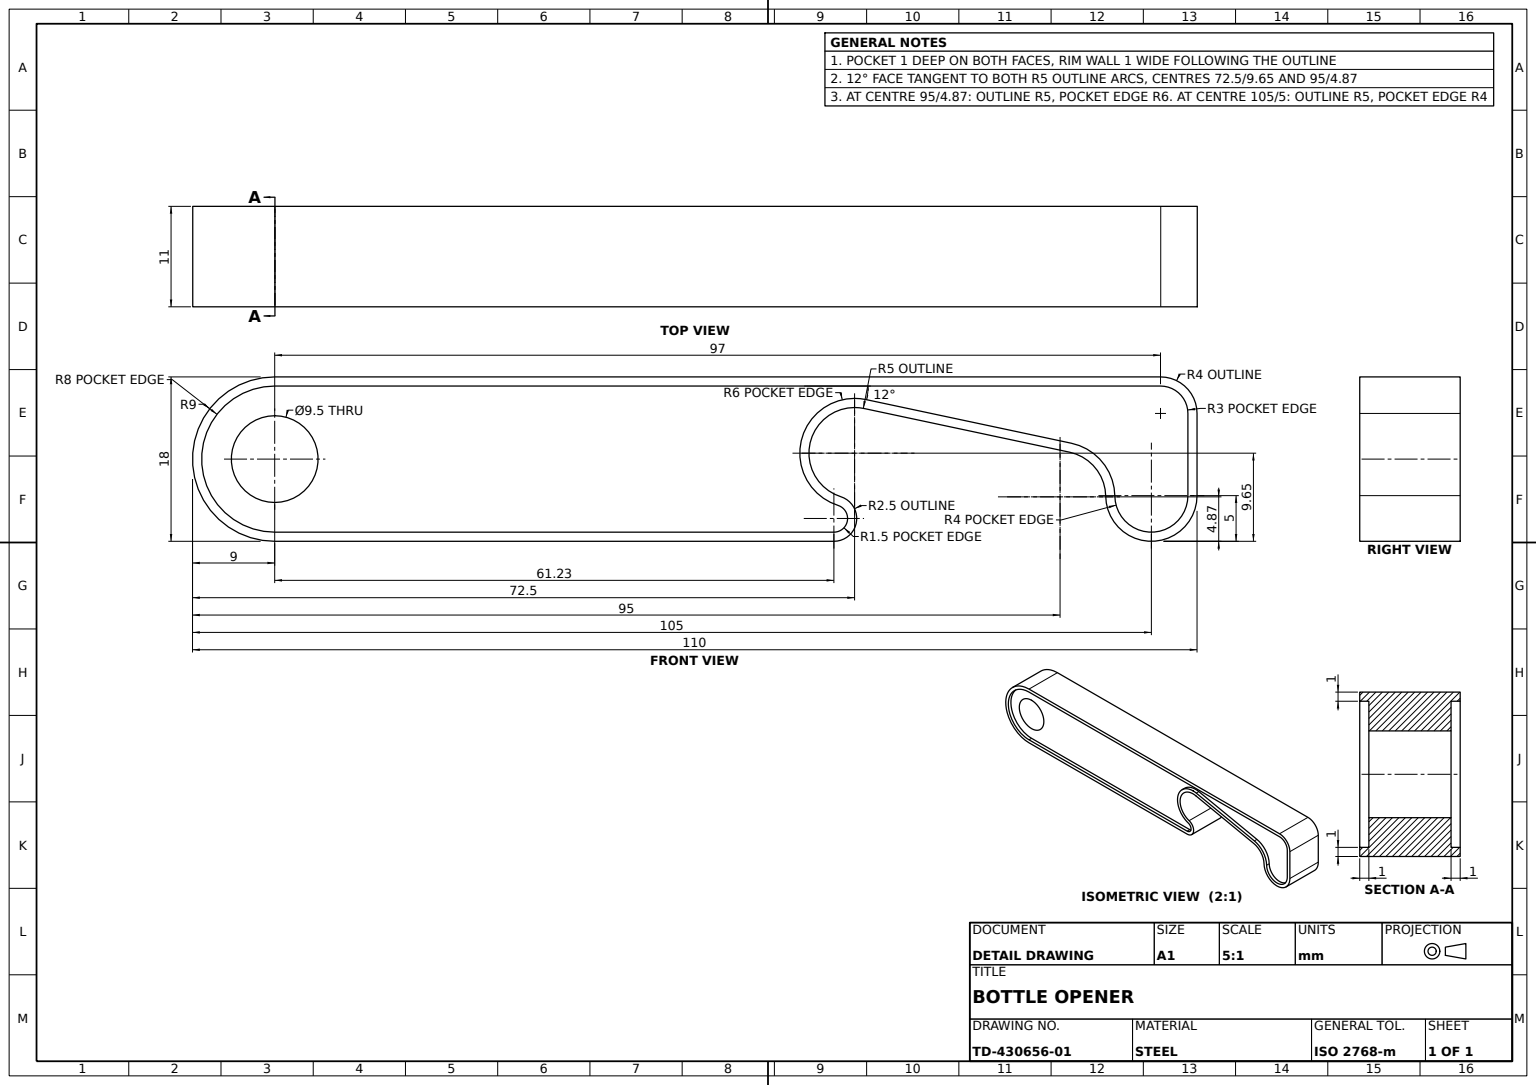
from build123d import *

# Parameters (mm, degrees)
OPENER_PROFILE_SKETCH_R = 4.75
OPENER_BODY_9MM_DEPTH   = 4.5
RAISED_RIM_11MM_DEPTH   = 5.5


with BuildPart() as part:
    # Opener Profile Sketch → Opener Body 9mm (new, symmetric)
    with BuildSketch(Plane(origin=(0, 0, 0), x_dir=(1, 0, 0), z_dir=(0, 1, 0))):
        with BuildLine():
            ThreePointArc((92.000354584, -4.053259235), (90.638520492, -0.326266085), (87.248356605, 1.735737516))
            Line((87.248356605, 1.735737516), (64.748356605, 6.518260154))
            ThreePointArc((64.748356605, 6.518260154), (57.699795888, 2.181480349), (61.687788593, -5.07012509))
            ThreePointArc((61.687788593, -5.07012509), (62.71687919, -6.72933342), (61.234514126, -8))
            Line((61.234514126, -8), (0, -8))
            ThreePointArc((0, -8), (-8, 0), (0, 8))
            Line((0, 8), (97, 8))
            ThreePointArc((97, 8), (99.121320344, 7.121320344), (100, 5))
            Line((100, 5), (100, -4))
            ThreePointArc((100, -4), (96.026630208, -7.999911353), (92.000354584, -4.053259235))
        make_face()
        with Locations(Location((0, 0, 0), (0, 0, 270))):
            Circle(OPENER_PROFILE_SKETCH_R, mode=Mode.SUBTRACT)
    extrude(amount=OPENER_BODY_9MM_DEPTH, both=True)

    # Sketch1_3 → Raised Rim 11mm (add, symmetric)
    with BuildSketch(Plane(origin=(0, 0, 0), x_dir=(1, 0, 0), z_dir=(0, 1, 0))):
        with BuildLine():
            ThreePointArc((91.00044323, -4.066574044), (89.865581487, -0.960746419), (87.040444914, 0.757589915))
            Line((87.040444914, 0.757589915), (64.540444914, 5.540112553))
            ThreePointArc((64.540444914, 5.540112553), (58.666644317, 1.926129382), (61.989971571, -4.11687515))
            ThreePointArc((61.989971571, -4.11687515), (63.705122566, -6.882222367), (61.234514126, -9))
            Line((61.234514126, -9), (0, -9))
            ThreePointArc((0, -9), (-9, 0), (0, 9))
            Line((0, 9), (97, 9))
            ThreePointArc((97, 9), (99.828427125, 7.828427125), (101, 5))
            Line((101, 5), (101, -4))
            ThreePointArc((101, -4), (96.03328776, -8.999889191), (91.00044323, -4.066574044))
        make_face()
        with BuildLine():
            ThreePointArc((92.000354584, -4.053259235), (96.026630208, -7.999911353), (100, -4))
            Line((100, -4), (100, 5))
            ThreePointArc((100, 5), (99.121320344, 7.121320344), (97, 8))
            Line((97, 8), (0, 8))
            ThreePointArc((0, 8), (-8, 0), (0, -8))
            Line((0, -8), (61.234514126, -8))
            ThreePointArc((61.234514126, -8), (62.71687919, -6.72933342), (61.687788593, -5.07012509))
            ThreePointArc((61.687788593, -5.07012509), (57.699795888, 2.181480349), (64.748356605, 6.518260154))
            Line((64.748356605, 6.518260154), (87.248356605, 1.735737516))
            ThreePointArc((87.248356605, 1.735737516), (90.638520492, -0.326266085), (92.000354584, -4.053259235))
        make_face(mode=Mode.SUBTRACT)
    extrude(amount=RAISED_RIM_11MM_DEPTH, both=True)


solid = part.part
